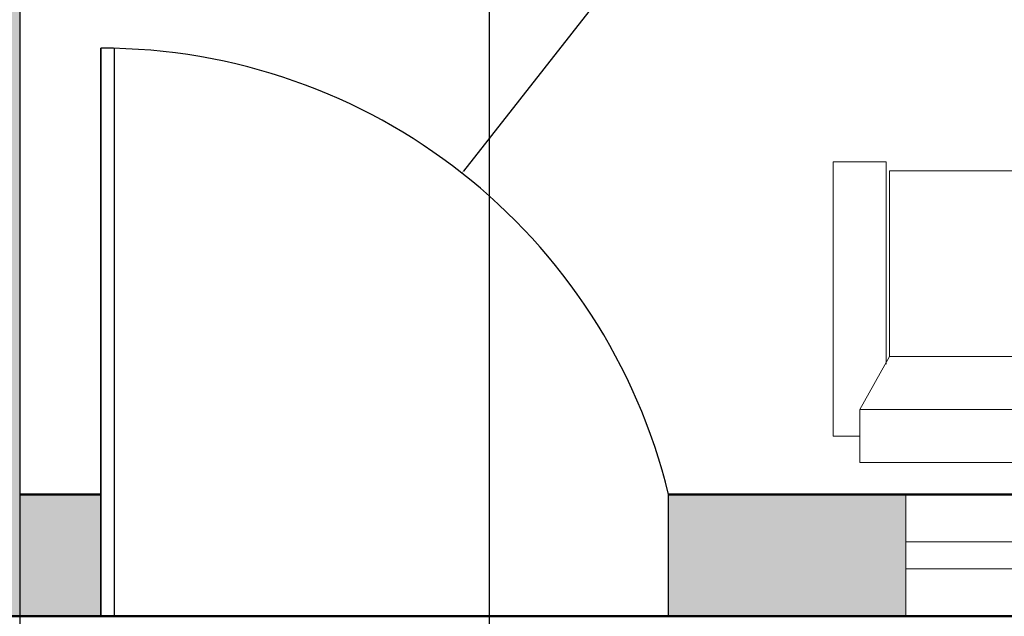
# Model space of a CAD drawing. Units: inches. Extents: x 3398 to 3816, y 15195 to 15771.
# Tile 4 of 10: x 3474 to 3547, y 15374 to 15418. Entities that reach past the tile are written whole.
import ezdxf

# ---------------------------------------------------------------- set-up
doc = ezdxf.new("R2010")
doc.units = ezdxf.units.IN
doc.header["$MEASUREMENT"] = 0
for name, color, linetype, lineweight in [('A-ANNO-DIMS', 2, 'Continuous', 18), ('A-DOOR', 3, 'Continuous', 25), ('A-FURN', 8, 'Continuous', 18), ('A-GLAZ', 4, 'Continuous', 18), ('A-WALL', 7, 'Continuous', 50), ('A-WALL-PATT', 252, 'Continuous', 13)]:
    doc.layers.add(name, color=color, linetype=linetype, lineweight=lineweight)
doc.styles.get("Standard").update_dxf_attribs({"font": 'arial.ttf'})
doc.dimstyles.get("Standard").update_dxf_attribs({"dimtxt": 6, "dimasz": 0.18, "dimexe": 0.18, "dimexo": 0.0625, "dimgap": 0.09, "dimtad": 0, "dimtih": 1, "dimtoh": 1, "dimdec": 1, "dimzin": 0, "dimdsep": 46, "dimlunit": 3, "dimtxsty": 'Standard', "dimcen": 0.09, "dimadec": 0, "dimazin": 0, "dimtfac": 1, "dimtdec": 1, "dimtofl": 0, "dimtmove": 0, "dimatfit": 3, "dimfxl": 1, "dimtolj": 1, "dimtzin": 0, "dimarcsym": 0})

# ---------------------------------------------------------------- blocks, each defined once
blk = doc.blocks.new('SOFA-3-SEAT')
for p, q in [((1.961, 55.044), (22.229, 55.044)), ((1.961, 55.044), (1.961, 53.083)), ((3.923, 55.044), (3.923, 1.962)), ((22.229, 51.121), (22.229, 55.044)), ((0, 53.083), (0, 1.962)), ((3.923, 53.083), (0, 53.083)), ((3.923, 53.083), (7.845, 50.876)), ((7.544, 51.121), (22.229, 51.121)), ((21.575, 50.874), (7.845, 50.874)), ((21.575, 35.305), (7.845, 35.305)), ((21.575, 19.737), (7.845, 19.737)), ((7.845, 4.168), (3.923, 1.962)), ((7.285, 3.923), (22.229, 3.923)), ((22.229, 3.923), (22.229, 0)), ((3.923, 1.962), (0, 1.962)), ((1.961, 1.962), (1.961, 0)), ((1.961, 0), (22.229, 0))]:
    blk.add_line(p, q)
blk.add_lwpolyline([(7.845, 50.876), (7.845, 4.168), (21.575, 4.168), (21.575, 50.874)])
blk = doc.blocks.new('WINDOW-SASH-48IN')
for p, q in [((48, 9), (0, 9)), ((48, 5.5), (0, 5.5)), ((0, 3.5), (48, 3.5)), ((0, 0), (48, 0))]:
    blk.add_line(p, q)
blk = doc.blocks.new('*D44')
at = {"layer": 'A-ANNO-DIMS', "color": 0, "lineweight": -2, "transparency": 16777216}
for p, q in [((3508.919, 15642.757), (3508.919, 15203.291)), ((3579.366, 15642.757), (3579.366, 15203.291)), ((3509.099, 15203.471), (3526.756, 15203.471)), ((3579.186, 15203.471), (3561.528, 15203.471))]:
    blk.add_line(p, q, dxfattribs=at)
at = {"layer": 'A-ANNO-DIMS', "color": 0, "transparency": 16777216}
for points in [[(3509.099, 15203.501), (3509.099, 15203.441), (3508.919, 15203.471)], [(3579.186, 15203.501), (3579.186, 15203.441), (3579.366, 15203.471)]]:
    blk.add_solid(points, dxfattribs=at)
at = {"layer": 'Defpoints', "color": 0, "transparency": 16777216}
for p in [(3508.919, 15642.82), (3579.366, 15642.82), (3579.366, 15203.471)]:
    blk.add_point(p, dxfattribs=at)
at = {"layer": 'A-ANNO-DIMS', "color": 0, "transparency": 16777216, "insert": (3544.142, 15203.471), "char_height": 6, "attachment_point": 5}
blk.add_mtext('\\A1;5\'-10 1/2"', dxfattribs=at)
blk = doc.blocks.new('*D53')
at = {"layer": 'A-ANNO-DIMS', "color": 0, "lineweight": -2, "transparency": 16777216}
for p, q in [((3508.919, 15642.757), (3508.919, 15203.291)), ((3474.189, 15601.458), (3474.189, 15203.291)), ((3474.369, 15203.471), (3508.739, 15203.471)), ((3508.919, 15203.471), (3509.099, 15203.471))]:
    blk.add_line(p, q, dxfattribs=at)
at = {"layer": 'A-ANNO-DIMS', "color": 0, "transparency": 16777216}
for points in [[(3474.369, 15203.501), (3474.369, 15203.441), (3474.189, 15203.471)], [(3508.739, 15203.501), (3508.739, 15203.441), (3508.919, 15203.471)]]:
    blk.add_solid(points, dxfattribs=at)
at = {"layer": 'Defpoints', "color": 0, "transparency": 16777216}
for p in [(3508.919, 15642.82), (3474.189, 15601.521), (3508.919, 15203.471)]:
    blk.add_point(p, dxfattribs=at)
at = {"layer": 'A-ANNO-DIMS', "color": 0, "transparency": 16777216, "insert": (3526.536, 15203.471), "char_height": 6, "attachment_point": 5}
blk.add_mtext('\\A1;2\'-10 1/2"', dxfattribs=at)
blk = doc.blocks.new('*D55')
at = {"layer": 'A-ANNO-DIMS', "color": 0, "lineweight": -2, "transparency": 16777216}
for p, q in [((3522.92, 15426.678), (3507.007, 15406.425)), ((3523.1, 15426.678), (3522.92, 15426.678)), ((3480.099, 15372.293), (3480.279, 15372.293)), ((3480.189, 15372.203), (3480.189, 15372.383))]:
    blk.add_line(p, q, dxfattribs=at)
at = {"layer": 'A-ANNO-DIMS', "color": 0, "transparency": 16777216}
blk.add_solid([(3506.983, 15406.444), (3507.031, 15406.407), (3506.896, 15406.284)], dxfattribs=at)
at = {"layer": 'Defpoints', "color": 0, "transparency": 16777216}
for p in [(3506.896, 15406.284), (3480.189, 15372.293)]:
    blk.add_point(p, dxfattribs=at)
at = {"layer": 'A-ANNO-DIMS', "color": 0, "transparency": 16777216, "insert": (3534.036, 15426.678), "char_height": 6, "attachment_point": 5}
blk.add_mtext('\\A1;R3\'-7"', dxfattribs=at)

msp = doc.modelspace()

# ---------------------------------------------------------------- hatches: boundary and pattern name
at = {"layer": 'A-WALL-PATT'}
h = msp.add_hatch(color=256, dxfattribs=at)
h.dxf.hatch_style = 1
h.paths.add_polyline_path([(3515.956, 15730.521), (3465.189, 15730.521), (3465.189, 15715.521), (3474.189, 15715.521), (3474.189, 15721.521), (3515.956, 15721.521)])
h.paths.add_polyline_path([(3719.807, 15730.521), (3675.765, 15730.521), (3675.765, 15721.521), (3700.689, 15721.521), (3700.689, 15637.521), (3610.689, 15637.521), (3610.689, 15663.972), (3606.189, 15663.972), (3606.189, 15601.521), (3599.084, 15601.521), (3599.084, 15592.521), (3606.189, 15592.521), (3606.189, 15508.521), (3616.689, 15508.521), (3616.689, 15513.021), (3610.689, 15513.021), (3610.689, 15633.021), (3708.189, 15633.021), (3708.189, 15637.521), (3705.189, 15637.521), (3705.189, 15721.521), (3719.807, 15721.521)])
h.paths.add_polyline_path([(3762.189, 15730.521), (3743.77, 15730.521), (3743.77, 15721.521), (3753.189, 15721.521), (3753.189, 15637.521), (3732.189, 15637.521), (3732.189, 15633.021), (3753.189, 15633.021), (3753.189, 15597.386), (3762.189, 15597.386)])
h.paths.add_polyline_path([(3762.189, 15549.386), (3753.189, 15549.386), (3753.189, 15513.021), (3652.689, 15513.021), (3652.689, 15508.521), (3664.689, 15508.521), (3664.689, 15460.521), (3652.689, 15460.521), (3652.689, 15456.021), (3672.189, 15456.021), (3672.189, 15460.521), (3669.189, 15460.521), (3669.189, 15508.521), (3753.189, 15508.521), (3753.189, 15497.511), (3762.189, 15497.511)])
h.paths.add_polyline_path([(3762.189, 15473.477), (3753.189, 15473.477), (3753.189, 15460.521), (3696.189, 15460.521), (3696.189, 15456.021), (3753.189, 15456.021), (3753.189, 15414.247), (3762.189, 15414.247)])
h.paths.add_polyline_path([(3762.189, 15366.279), (3753.189, 15366.279), (3753.189, 15324.021), (3610.689, 15324.021), (3610.689, 15456.021), (3616.689, 15456.021), (3616.689, 15460.521), (3610.689, 15460.521), (3606.189, 15460.521), (3606.189, 15382.521), (3587.73, 15382.521), (3587.73, 15373.521), (3606.189, 15373.521), (3606.189, 15315.021), (3762.189, 15315.021)])
h.paths.add_polyline_path([(3539.73, 15382.521), (3522.189, 15382.521), (3522.189, 15373.521), (3539.73, 15373.521)])
h.paths.add_polyline_path([(3480.189, 15382.521), (3474.189, 15382.521), (3474.189, 15452.469), (3465.189, 15452.469), (3465.189, 15373.521), (3480.189, 15373.521)])
h.paths.add_polyline_path([(3551.043, 15601.521), (3474.189, 15601.521), (3474.189, 15679.521), (3465.189, 15679.521), (3465.189, 15500.469), (3474.189, 15500.469), (3474.189, 15592.521), (3551.043, 15592.521)])

# ---------------------------------------------------------------- linework, layer by layer
at = {"layer": 'A-DOOR'}
for p, q in [((3480.189, 15409.521), (3480.189, 15415.521)), ((3480.189, 15415.521), (3480.189, 15373.521)), ((3481.189, 15415.521), (3481.189, 15373.521)), ((3480.189, 15373.521), (3480.189, 15409.521)), ((3522.189, 15373.521), (3522.189, 15382.521)), ((3474.189, 15373.521), (3480.189, 15373.521)), ((3480.189, 15373.521), (3522.189, 15373.521))]:
    msp.add_line(p, q, dxfattribs=at)
msp.add_arc((3480.189, 15372.293), 43.227, 13.68555, 90, dxfattribs=at)
at = {"layer": 'A-GLAZ'}
msp.add_line((3539.73, 15373.521), (3539.73, 15382.521), dxfattribs=at)
at = {"layer": 'A-WALL'}
for p, q in [((3474.189, 15382.521), (3480.189, 15382.521)), ((3522.189, 15382.521), (3606.189, 15382.521)), ((3465.189, 15373.521), (3606.189, 15373.521))]:
    msp.add_line(p, q, dxfattribs=at)

# ---------------------------------------------------------------- block references
at = {"layer": 'A-FURN', "extrusion": (0, 0, -1), "zscale": -1, "rotation": 90.00000000000078}
msp.add_blockref('SOFA-3-SEAT', (-3534.368, 15384.878), dxfattribs=at)
at = {"layer": 'A-GLAZ', "rotation": 180}
msp.add_blockref('WINDOW-SASH-48IN', (3587.73, 15382.52), dxfattribs=at)

# ---------------------------------------------------------------- dimensions: what is measured, and where the dimension line sits
at = {"layer": 'A-ANNO-DIMS'}
for base, p1, p2, picture, middle in [((3508.919, 15203.471), (3474.189, 15601.521), (3508.919, 15642.82), '*D53', (3526.536, 15203.471)), ((3579.366, 15203.471), (3508.919, 15642.82), (3579.366, 15642.82), '*D44', (3544.142, 15203.471))]:
    dim = msp.add_linear_dim(base=base, p1=p1, p2=p2, dimstyle='Standard', override={"dimdec": 1, "dimlfac": 1, "dimrnd": 0, "dimzin": 1, "dimdsep": 46, "dimlunit": 4, "dimfrac": 2}, dxfattribs=at)
    dim.commit()
    dim.dimension.update_dxf_attribs({"geometry": picture, "text_midpoint": middle})
dim = msp.add_radius_dim(center=(3480.189, 15372.293), mpoint=(3506.896, 15406.284), dimstyle='Standard', override={"dimdec": 1, "dimlfac": 1, "dimrnd": 0, "dimzin": 1, "dimdsep": 46, "dimlunit": 4, "dimfrac": 2}, dxfattribs=at)
dim.commit()
dim.dimension.update_dxf_attribs({"geometry": '*D55', "text_midpoint": (3534.036, 15426.678), "dimtype": 164})

doc.saveas('drawing.dxf')
